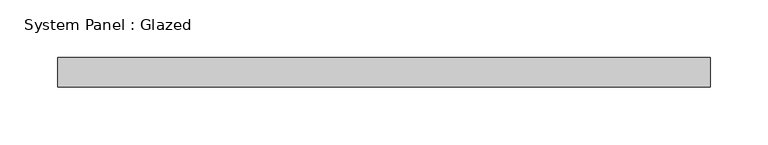
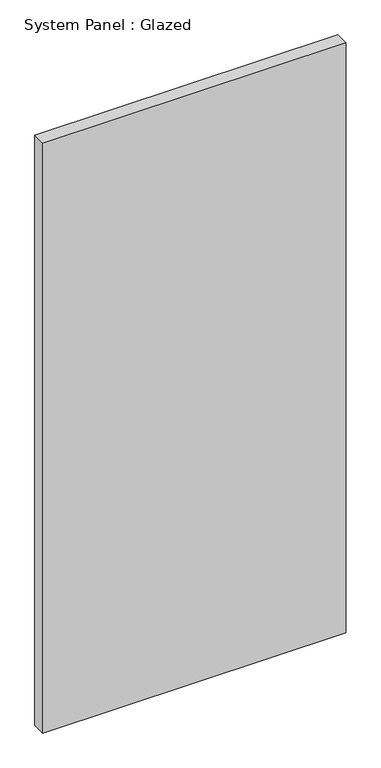
"""IFC4 building model written with IfcOpenShell, lengths in millimetres: plate geometry, System Panel : Glazed."""

from ifc_helpers import new_model, si_unit, origin, origin_with_axes, place, context, project, spatial, polyline, outline, extrude, source, transform, mapped, element, save


def system_panel_glazed_ed2f53c1(model_context):
    return source(origin(), model_context, "Body", "SweptSolid", [
        extrude(outline(polyline([(282.575, 19.05), (-282.575, 19.05), (-282.575, 44.45), (282.575, 44.45), (282.575, 19.05)])), origin_with_axes(), (0.0, 0.0, 1.0), 1161.9615505),
    ])


if __name__ == "__main__":
    model = new_model("IFC4")
    model_context = context("Model", 3, world=origin())
    ifc_project = project(units=[si_unit("LENGTHUNIT", "METRE", prefix="MILLI")], contexts=[model_context])
    site = spatial("IfcSite", under=ifc_project)
    building = spatial("IfcBuilding", under=site)
    placement = place(None, origin())
    system_panel_glazed_shape = system_panel_glazed_ed2f53c1(model_context)
    element("IfcPlate", 1, ObjectType="System Panel : Glazed", at=placement, inside=building, context=model_context, shape_type="MappedRepresentation", body=[
        mapped(system_panel_glazed_shape, transform((0.0, 0.0, 0.0), x_axis=(1.0, 0.0, 0.0), y_axis=(0.0, 1.0, 0.0), z_axis=(0.0, 0.0, 1.0))),
    ])
    save(model, "model.ifc")

# Revit data of these elements
# Type "System Panel : Glazed"
#   Construction Type Id = "GSP4R"
#   Analytic Construction = "1/8 in Pilkington single glazing"
#   Visual Light Transmittance = 0.9
#   Solar Heat Gain Coefficient = 0.86
#   Heat Transfer Coefficient (U) = 1.18115 BTU/(h·ft²·°F)
#   Define Thermal Properties by = 1
# Element 1 (IfcPlate, "System Panel : Glazed")
#   Materials on its faces: "Glass"
# Materials
#   "Glass": class "Glass", colour RGB 0 128 192, transparency 0.75, Description = "Soda Lime Glass", Cost = 0
